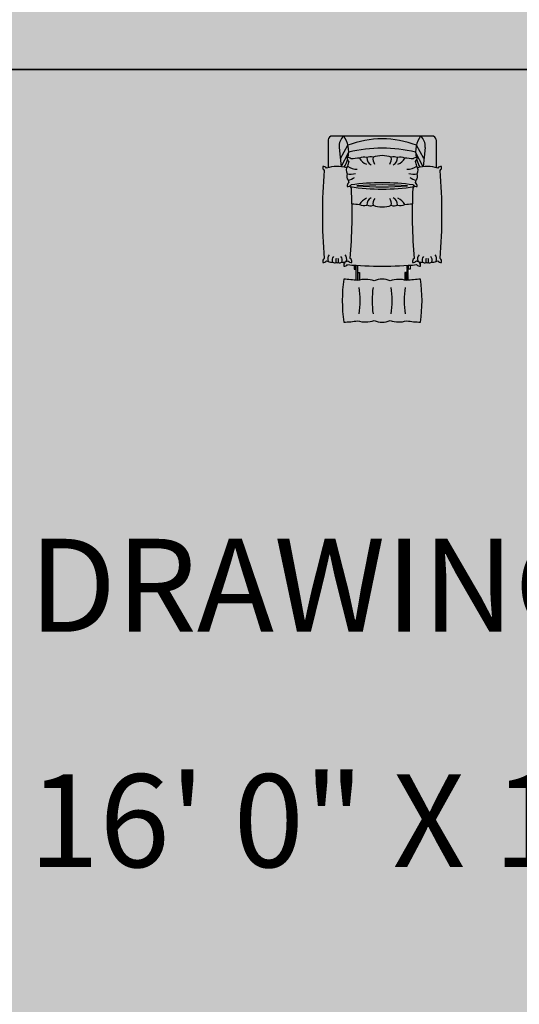
# Model space of a CAD drawing. Units: inches. Extents: x 1704 to 6393, y -157 to 1172.
# Tile 21 of 122: x 2087 to 2161, y 227 to 372. Entities that reach past the tile are written whole.
import ezdxf

# ---------------------------------------------------------------- set-up
doc = ezdxf.new("R2010")
doc.units = ezdxf.units.IN
doc.header["$MEASUREMENT"] = 0
for name, color, linetype, lineweight in [('A-ANNO-DIMS', 7, 'Continuous', 13), ('A-AREA-IDEN', 7, 'Continuous', 18), ('A-FURN', 8, 'Continuous', 18), ('A-WALL-PATT', 7, 'Continuous', 13), ('estofado', 7, 'Continuous', 25), ('WALLS', 7, 'Continuous', 35)]:
    doc.layers.add(name, color=color, linetype=linetype, lineweight=lineweight)
doc.layers.add('A-FLOR-PATT', color=7, linetype='Continuous', lineweight=13, true_color=0xf2f2f2)
doc.styles.get("Standard").update_dxf_attribs({"font": 'arial.ttf'})
doc.dimstyles.get("Standard").update_dxf_attribs({"dimtxt": 6, "dimasz": 2, "dimexe": 0.18, "dimexo": 0.0625, "dimgap": 0.09, "dimtad": 0, "dimtih": 1, "dimtoh": 1, "dimdec": 1, "dimzin": 0, "dimdsep": 46, "dimlunit": 3, "dimtxsty": 'Standard', "dimblk": 'ARCHTICK', "dimcen": 0.09, "dimadec": 0, "dimazin": 0, "dimtfac": 1, "dimtdec": 1, "dimtofl": 0, "dimtmove": 0, "dimatfit": 3, "dimfxl": 1, "dimtolj": 1, "dimtzin": 0, "dimarcsym": 0})

# ---------------------------------------------------------------- blocks, each defined once
blk = doc.blocks.new('Poltrona Del Rey Aliança')
at = {"layer": 'estofado', "ltscale": 0.1}
h = blk.add_hatch(color=256, dxfattribs=at)
h.dxf.hatch_style = 1
h.set_gradient(color1=(204, 209, 209), color2=(140, 151, 151), one_color=1, tint=0.57, name='CYLINDER')
h.paths.add_polyline_path([(-0.3291, -0.0872, -0.258328), (-0.295, 0), (-0.3837, 0, 0.414214), (-0.4137, -0.03), (-0.4137, -0.2425, -0.088666), (-0.3154, -0.2356)])
h.paths.add_polyline_path([(0.4137, -0.03, 0.414214), (0.3837, 0), (0.295, 0, -0.258328), (0.3291, -0.0872), (0.3154, -0.2356, -0.088666), (0.4137, -0.2425)])
h = blk.add_hatch(color=256, dxfattribs=at)
h.dxf.hatch_style = 1
h.set_gradient(color1=(204, 209, 209), color2=(140, 151, 151), one_color=1, tint=0.57, name='INVCYLINDER')
h.paths.add_polyline_path([(0.295, 0), (-0.295, 0, -0.089046), (-0.2635, -0.0705, -0.183028), (0.2635, -0.0705, -0.089046)])
h = blk.add_hatch(color=256, dxfattribs=at)
h.dxf.hatch_style = 1
h.set_gradient(color1=(204, 209, 209), color2=(140, 151, 151), one_color=1, tint=0.57)
h.paths.add_polyline_path([(-0.2635, -0.0705, 0.089046), (-0.295, 0, 0.258328), (-0.3291, -0.0872), (-0.3212, -0.1727)])
h.paths.add_polyline_path([(-0.2571, -0.1231, 0.060804), (-0.2635, -0.0705), (-0.3212, -0.1727), (-0.3154, -0.2356)])
h.paths.add_polyline_path([(-0.2655, -0.1833, -0.142988), (-0.2685, -0.1646, -0.055221), (-0.261, -0.1645, 0.047677), (-0.2571, -0.1231), (-0.3154, -0.2356, -0.022481), (-0.2906, -0.2393, 0.070542)])
h = blk.add_hatch(color=256, dxfattribs=at)
h.dxf.hatch_style = 1
h.set_gradient(color1=(204, 209, 209), color2=(140, 151, 151), one_color=1, tint=0.57, name='INVCYLINDER')
h.paths.add_polyline_path([(-0.2635, -0.0705, -0.060804), (-0.2571, -0.1231, -0.113324), (0.2571, -0.1231, -0.060804), (0.2635, -0.0705, 0.183028)])
h = blk.add_hatch(color=256, dxfattribs=at)
h.dxf.hatch_style = 1
h.set_gradient(color1=(204, 209, 209), color2=(140, 151, 151), one_color=1, tint=0.57)
h.paths.add_polyline_path([(0.295, 0, 0.089046), (0.2635, -0.0705), (0.3211, -0.1738), (0.3291, -0.0872, 0.258328)])
h.paths.add_polyline_path([(0.2635, -0.0705, 0.060804), (0.2571, -0.1231), (0.3154, -0.2356), (0.3211, -0.1738)])
h.paths.add_polyline_path([(0.2571, -0.1231, 0.047677), (0.261, -0.1645, -0.055221), (0.2685, -0.1646, -0.142988), (0.2655, -0.1833, 0.070542), (0.2906, -0.2393, -0.022481), (0.3154, -0.2356)])
h = blk.add_hatch(color=256, dxfattribs=at)
h.dxf.hatch_style = 1
h.set_gradient(color1=(204, 209, 209), color2=(85, 94, 94), one_color=1, tint=0.35, name='CURVED')
h.paths.add_polyline_path([(-0.2568, -0.1947, -0.107782), (-0.2655, -0.1833, -0.070542), (-0.2906, -0.2393, -0.016789), (-0.2722, -0.2436, -0.067663), (-0.2652, -0.2308, -0.033072)])
h.paths.add_polyline_path([(0.2571, -0.1231, 0.113324), (-0.2571, -0.1231, -0.047677), (-0.261, -0.1645, -0.196708), (-0.2383, -0.1763, -0.00792), (-0.1747, -0.1697, -0.182617), (-0.118, -0.1656, -0.204275), (-0.0697, -0.1634, -0.180654), (0.0697, -0.1634, -0.204275), (0.118, -0.1656, -0.182617), (0.1747, -0.1697, -0.00792), (0.2383, -0.1763, -0.196708), (0.261, -0.1645, -0.047677)])
h.paths.add_polyline_path([(0.2655, -0.1833, -0.107782), (0.2568, -0.1947, -0.033072), (0.2652, -0.2308, -0.067663), (0.2722, -0.2436, -0.016789), (0.2906, -0.2393, -0.070542)])
h = blk.add_hatch(color=256, dxfattribs=at)
h.dxf.hatch_style = 1
h.set_gradient(color1=(204, 209, 209), color2=(140, 151, 151), one_color=1, tint=0.57, name='INVCURVED')
h.paths.add_polyline_path([(0.2652, -0.2308, 0.033072), (0.2568, -0.1947, 0.254696), (0.2685, -0.1646, 0.254696), (0.2383, -0.1763, 0.00792), (0.1747, -0.1697, 0.182617), (0.118, -0.1656, 0.187401), (0.0735, -0.1621, 0.016251), (0.0697, -0.1634, 0.180654), (-0.0697, -0.1634, 0.204275), (-0.118, -0.1656, 0.263328), (-0.0893, -0.2185, -0.263328), (-0.118, -0.1656, 0.182617), (-0.1747, -0.1697, 0.00792), (-0.2383, -0.1763, 0.254696), (-0.2685, -0.1646, 0.254696), (-0.2568, -0.1947, 0.033072), (-0.2652, -0.2308, 0.299987), (-0.2685, -0.2905, 0.296972), (-0.2615, -0.3402, 0.016266), (-0.2568, -0.3578, 0.254696), (-0.2685, -0.388, 0.254696), (-0.2383, -0.3763, -0.073513), (0.2383, -0.3763, 0.254696), (0.2685, -0.388, 0.254696), (0.2568, -0.3578, 0.016266), (0.2615, -0.3402, 0.296972), (0.2685, -0.2905, 0.299987)])
h = blk.add_hatch(color=256, dxfattribs=at)
h.dxf.hatch_style = 1
h.set_gradient(color1=(204, 209, 209), one_color=1, tint=1)
h.paths.add_polyline_path([(-0.2358, -0.4039, 0.314303), (-0.2519, -0.386, -0.125347), (-0.2685, -0.388, -0.254696), (-0.2568, -0.3578, -0.016266), (-0.2615, -0.3402, -0.296972), (-0.2685, -0.2905, -0.227702), (-0.2722, -0.2436, 0.140506), (-0.4265, -0.2461, 0.254696), (-0.4567, -0.2344, 0.254696), (-0.445, -0.2646, 0.041763), (-0.445, -0.9409, 0.254696), (-0.4567, -0.971, 0.254696), (-0.4265, -0.9594, 0.011584), (-0.414, -0.9628, 0.212443), (-0.3803, -0.9693, 0.2364), (-0.3527, -0.9714, 0.216836), (-0.3417, -0.9734, 0.091294), (-0.3373, -0.9714, 0.2364), (-0.3097, -0.9693, 0.284493), (-0.3149, -0.9268, -0.284493), (-0.3097, -0.9693, 0.212443), (-0.276, -0.9628, 0.011584), (-0.2635, -0.9594, 0.254696), (-0.2333, -0.971, 0.254696), (-0.245, -0.9409, 0.033141)])
h = blk.add_hatch(color=256, dxfattribs=at)
h.dxf.hatch_style = 1
h.set_gradient(color1=(204, 209, 209), one_color=1, tint=1)
h.paths.add_polyline_path([(0.445, -0.2646, 0.254696), (0.4567, -0.2344, 0.254696), (0.4265, -0.2461, 0.140506), (0.2722, -0.2436, -0.227702), (0.2685, -0.2905, -0.296972), (0.2615, -0.3402, -0.016266), (0.2568, -0.3578, -0.254696), (0.2685, -0.388, -0.125347), (0.2519, -0.386, 0.314303), (0.2358, -0.4039, 0.033141), (0.245, -0.9409, 0.254696), (0.2333, -0.971, 0.254696), (0.2635, -0.9594, 0.011584), (0.276, -0.9628, 0.212443), (0.3097, -0.9693, 0.2364), (0.3373, -0.9714, 0.314353), (0.3527, -0.9714, 0.2364), (0.3803, -0.9693, 0.212443), (0.414, -0.9628, 0.011584), (0.4265, -0.9594, 0.254696), (0.4567, -0.971, 0.254696), (0.445, -0.9409, 0.041763)])
h = blk.add_hatch(color=256, dxfattribs=at)
h.dxf.hatch_style = 1
h.set_gradient(color1=(204, 209, 209), color2=(140, 151, 151), one_color=1, tint=0.57, name='INVCURVED')
h.paths.add_polyline_path([(-0.2383, -0.3763, -0.125347), (-0.2519, -0.386, -0.093275), (-0.2447, -0.3891, 0.075524), (0.2447, -0.3891, -0.093275), (0.2519, -0.386, -0.125347), (0.2383, -0.3763, 0.073513)])
h.paths.add_polyline_path([(0.1958, -0.3832, -0.03688), (-0.1958, -0.3832, -0.03688)], flags=16)
h = blk.add_hatch(color=256, dxfattribs=at)
h.dxf.hatch_style = 1
h.set_gradient(color1=(204, 209, 209), color2=(129, 141, 141), one_color=1, tint=0.53, name='CURVED')
h.paths.add_polyline_path([(0.2356, -0.4071, -0.253895), (0.2447, -0.3891, -0.075524), (-0.2447, -0.3891, -0.253895), (-0.2356, -0.4071, -0.006973), (-0.2317, -0.5201, 0.007144), (-0.1744, -0.5259, -0.00012), (-0.1743, -0.5259, 0.182617), (-0.1176, -0.53, 0.204275), (-0.0693, -0.5322, 0.180654), (0.0701, -0.5322, 0.204275), (0.1184, -0.53, 0.182617), (0.1751, -0.5259, 0.000052), (0.1751, -0.5258, 0.00705), (0.2317, -0.5201, -0.006973)])
h = blk.add_hatch(color=256, dxfattribs=at)
h.dxf.hatch_style = 1
h.set_gradient(color1=(204, 209, 209), one_color=1, tint=1, name='CYLINDER')
h.paths.add_polyline_path([(0.2317, -0.5201, -0.007042), (0.1752, -0.5258, -0.182811), (0.1184, -0.53, -0.204275), (0.0701, -0.5322, -0.180542), (-0.0693, -0.5323, -0.000018), (-0.0694, -0.5323, -0.203561), (-0.1175, -0.53, -0.000024), (-0.1177, -0.53, -0.181815), (-0.1742, -0.5259, -0.007163), (-0.2317, -0.5201, -0.025969), (-0.245, -0.9409, -0.254696), (-0.2333, -0.971, -0.254696), (-0.2635, -0.9594, -0.011584), (-0.276, -0.9628, -0.070407), (-0.2865, -0.9682, 0.130579), (-0.295, -0.9977), (-0.295, -1, 0.254696), (-0.2648, -0.9883, 0.044151), (0.2648, -0.9883, 0.254696), (0.295, -1), (0.295, -0.9977, 0.130579), (0.2865, -0.9682, -0.070407), (0.276, -0.9628, -0.011584), (0.2635, -0.9594, -0.254696), (0.2333, -0.971, -0.254696), (0.245, -0.9409, -0.025969)])
h = blk.add_hatch(color=256, dxfattribs=at)
h.dxf.hatch_style = 1
h.set_gradient(color1=(204, 209, 209), one_color=1, tint=1, name='CYLINDER')
h.paths.add_polyline_path([(0.295, -1.0999, 0.031185), (0.1884, -1.1106, 0.17196), (0.0623, -1.1138, 0.223433), (-0.0623, -1.1138, 0.17196), (-0.1884, -1.1106, 0.031185), (-0.295, -1.0999, 0.066975), (-0.295, -1.43, 0.031185), (-0.1884, -1.4193, 0.17196), (-0.0623, -1.4161, 0.223433), (0.0623, -1.4161, 0.17196), (0.1884, -1.4193, 0.031185), (0.295, -1.43, 0.066975)])
at = {"layer": 'estofado'}
for p, q in [((0.3837, 0), (-0.3837, 0)), ((-0.4137, -0.03), (-0.4137, -0.2425)), ((0.4137, -0.03), (0.4137, -0.2425)), ((-0.3291, -0.0872), (-0.3154, -0.2356)), ((0.3291, -0.0872), (0.3154, -0.2356)), ((-0.295, -0.9701), (-0.295, -1)), ((0.295, -1), (0.295, -0.9701))]:
    blk.add_line(p, q, dxfattribs=at)
at = {"layer": 'estofado', "ltscale": 0.1}
for p, q in [((-0.3212, -0.1727), (-0.2635, -0.0705)), ((0.3211, -0.1738), (0.2635, -0.0705)), ((-0.3154, -0.2356), (-0.2571, -0.1231)), ((0.3154, -0.2356), (0.2571, -0.1231))]:
    blk.add_line(p, q, dxfattribs=at)
for points in [[(-0.2141, -0.9924), (-0.2141, -1.0234), (-0.2033, -1.0234), (-0.2033, -0.9931)], [(-0.2003, -1.1087), (-0.2003, -0.9933)], [(-0.1897, -0.994), (-0.1897, -1.1104)], [(-0.1852, -1.1096), (-0.1852, -1.0474), (-0.1745, -1.0474), (-0.1745, -1.1066)], [(0.1852, -1.1096), (0.1852, -1.0474), (0.1745, -1.0474), (0.1745, -1.1066)], [(0.1897, -0.994), (0.1897, -1.1104)], [(0.2003, -1.1087), (0.2003, -0.9933)], [(0.2141, -0.9924), (0.2141, -1.0234), (0.2033, -1.0234), (0.2033, -0.9931)]]:
    blk.add_lwpolyline(points, dxfattribs=at)
at = {"layer": 'estofado'}
for centre, radius, start, end in [((-0.3837, -0.03), 0.03, 90, 180), ((-0.2333, -0.0744), 0.0967, 129.65366, 187.59148), ((-0.4756, -0.1231), 0.2185, 349.08151, 34.27248), ((0.4756, -0.1231), 0.2185, 145.72752, 190.91849), ((0.2333, -0.0744), 0.0967, 352.40852, 50.34634), ((0.3837, -0.03), 0.03, 360, 90), ((-0.4756, -0.1231), 0.2185, 327.85602, 343.99631), ((-0.2349, -0.1689), 0.0338, 172.61866, 229.77535), ((-0.2641, -0.1981), 0.0338, 40.22465, 97.38134), ((0.0111, -0.2763), 0.28, 163.06826, 170.64501), ((0, -2.1798), 2.0176, 94.96806, 96.78307), ((0, -2.1798), 2.0176, 83.21693, 85.03194), ((0.2641, -0.1981), 0.0338, 82.61866, 139.77535), ((0.2349, -0.1689), 0.0338, 310.22465, 7.38134), ((-0.0111, -0.2763), 0.28, 9.35499, 16.93174), ((0.4756, -0.1231), 0.2185, 196.00369, 212.14398), ((3.5965, -0.6027), 4.0556, 175.21711, 184.78289), ((-0.4232, -0.2388), 0.0338, 172.61866, 229.77535), ((-0.4524, -0.268), 0.0338, 40.22465, 97.38134), ((-0.345, -0.514), 0.28, 74.93962, 106.93174), ((-0.2215, -0.2632), 0.0544, 143.38498, 210.17914), ((-0.2269, -0.31), 0.046, 154.98172, 221.1415), ((0.2269, -0.31), 0.046, 318.8585, 25.01828), ((0.2215, -0.2632), 0.0544, 329.82086, 36.61502), ((0.345, -0.514), 0.28, 73.06826, 105.06038), ((0.4524, -0.268), 0.0338, 82.61866, 139.77535), ((0.4232, -0.2388), 0.0338, 310.22465, 7.38134), ((-3.5965, -0.6027), 4.0556, 355.21711, 4.78289), ((-0.2349, -0.3836), 0.0338, 130.22465, 187.38134), ((-0.2641, -0.3545), 0.0338, 262.61866, 319.77535), ((0.0111, -0.2763), 0.28, 193.20412, 196.93174), ((0, -3.0337), 2.6577, 85.77582, 94.22418), ((0.2641, -0.3545), 0.0338, 220.22465, 277.38134), ((-0.0111, -0.2763), 0.28, 343.06826, 346.79588), ((0.2349, -0.3836), 0.0338, 352.61866, 49.77535), ((-0.2567, -0.4065), 0.0211, 358.53397, 76.83372), ((-4.2865, -0.6027), 4.0556, 355.21711, 2.80978), ((0, 2.2673), 2.6577, 265.77582, 274.22418), ((4.2865, -0.6027), 4.0556, 177.19022, 184.78289), ((0.2567, -0.4065), 0.0211, 103.16628, 181.46603), ((0, 1.4842), 2.0176, 263.40516, 265.04688), ((0, 1.4842), 2.0176, 274.97902, 276.59484), ((0, 1.4842), 2.0176, 266.65527, 266.66071), ((0, 1.4842), 2.0176, 268.02834, 268.03255), ((-0.4232, -0.9667), 0.0338, 130.22465, 187.38134), ((-0.4524, -0.9375), 0.0338, 262.61866, 319.77535), ((-0.345, -0.6915), 0.28, 253.06826, 255.723), ((-0.2353, -0.9988), 0.0598, 149.12344, 181.11851), ((-0.345, -0.6915), 0.28, 284.277, 286.93174), ((-0.2376, -0.9375), 0.0338, 220.22465, 277.38134), ((-0.2668, -0.9667), 0.0338, 352.61866, 49.77535), ((0.2668, -0.9667), 0.0338, 130.22465, 187.38134), ((0.2376, -0.9375), 0.0338, 262.61866, 319.77535), ((0.345, -0.6915), 0.28, 253.06826, 255.723), ((0.2353, -0.9988), 0.0598, 358.88149, 30.87656), ((0.345, -0.6915), 0.28, 284.277, 286.93174), ((0.4524, -0.9375), 0.0338, 220.22465, 277.38134), ((0.4232, -0.9667), 0.0338, 352.61866, 49.77535), ((-0.2907, -0.9665), 0.0338, 262.61866, 319.77535), ((0, 2.0052), 3.0052, 264.94391, 275.05609), ((0.2907, -0.9665), 0.0338, 220.22465, 277.38134)]:
    blk.add_arc(centre, radius, start, end, dxfattribs=at)
at = {"layer": 'estofado', "ltscale": 0.1}
for centre, radius, start, end in [((0, -0.7661), 0.7439, 69.25617, 110.74383), ((0, -1.2427), 1.1487, 77.06919, 102.93081), ((0, -0.3501), 0.1993, 69.51952, 110.48048), ((-0.1409, -0.2427), 0.0805, 73.46231, 114.85878), ((-0.0792, -0.1148), 0.1102, 209.89617, 247.80825), ((-0.0912, -0.2211), 0.0616, 69.57655, 115.75748), ((-0.057, -0.1667), 0.061, 178.98456, 242.48365), ((-0.0035, -0.1761), 0.0675, 169.12551, 216.59576), ((0.0035, -0.1761), 0.0675, 323.40424, 10.87449), ((0.0912, -0.2211), 0.0616, 64.24252, 110.42345), ((0.057, -0.1667), 0.061, 297.51635, 1.01544), ((0.1409, -0.2427), 0.0805, 65.14122, 106.53769), ((0.0792, -0.1148), 0.1102, 292.19175, 330.10383), ((-0.2431, -0.1831), 0.1104, 256.68043, 289.83371), ((-0.2036, -0.1635), 0.0913, 227.53176, 278.05529), ((0.2036, -0.1635), 0.0913, 261.94471, 312.46824), ((0.2431, -0.1831), 0.1104, 250.16629, 283.31957), ((-0.3064, -0.1722), 0.1739, 284.94614, 302.97426), ((0, -1.9883), 1.6296, 81.59117, 98.40883), ((0.3064, -0.1722), 0.1739, 237.02574, 255.05386), ((0, 1.222), 1.6296, 261.36198, 278.63802), ((-0.0788, -0.5808), 0.1102, 112.19175, 150.10383), ((-0.1405, -0.4529), 0.0805, 245.14122, 286.53769), ((-0.0566, -0.5289), 0.061, 117.51635, 181.01544), ((-0.0031, -0.5195), 0.0675, 143.40424, 190.87449), ((0.0039, -0.5195), 0.0675, 349.12551, 36.59576), ((0.0574, -0.5289), 0.061, 358.98456, 62.48365), ((0.1413, -0.4529), 0.0805, 253.46231, 294.85878), ((0.0796, -0.5808), 0.1102, 29.89617, 67.80825), ((-0.0908, -0.4745), 0.0616, 244.24252, 290.42345), ((0.0004, -0.3455), 0.1993, 249.51952, 290.48048), ((0.0916, -0.4745), 0.0616, 249.57655, 295.75748), ((-0.369, -0.9438), 0.0489, 140.1555, 202.877), ((-0.3899, -0.9281), 0.0423, 235.25652, 283.23173), ((-0.3434, -0.9522), 0.0406, 137.80589, 204.86284), ((-0.3644, -0.9429), 0.0308, 238.98878, 292.19094), ((-0.3124, -0.9555), 0.0434, 159.33684, 201.47674), ((-0.345, -0.9603), 0.0135, 235.09864, 304.90136), ((-0.3776, -0.9555), 0.0434, 338.52326, 20.66316), ((-0.3256, -0.9429), 0.0308, 247.80906, 301.01122), ((-0.3466, -0.9522), 0.0406, 335.13716, 42.19411), ((-0.3001, -0.9281), 0.0423, 256.76827, 304.74348), ((-0.321, -0.9438), 0.0489, 337.123, 39.8445), ((0.321, -0.9438), 0.0489, 140.1555, 202.877), ((0.3001, -0.9281), 0.0423, 235.25652, 283.23173), ((0.3466, -0.9522), 0.0406, 137.80589, 204.86284), ((0.3256, -0.9429), 0.0308, 238.98878, 292.19094), ((0.3776, -0.9555), 0.0434, 159.33684, 201.47674), ((0.345, -0.9603), 0.0135, 235.09864, 304.90136), ((0.3124, -0.9555), 0.0434, 338.52326, 20.66316), ((0.3644, -0.9429), 0.0308, 247.80906, 301.01122), ((0.3434, -0.9522), 0.0406, 335.13716, 42.19411), ((0.3899, -0.9281), 0.0423, 256.76827, 304.74348), ((0.369, -0.9438), 0.0489, 337.123, 39.8445), ((0.9317, -1.2649), 1.2378, 172.33668, 187.66332), ((-0.3276, -1.9587), 0.8594, 80.68246, 87.82718), ((-0.1299, -1.2902), 0.1889, 69.03471, 108.06338), ((0, -1.2462), 0.1463, 64.81025, 115.18975), ((0.1299, -1.2902), 0.1889, 71.93662, 110.96529), ((0.3276, -1.9587), 0.8594, 92.17282, 99.31754), ((-0.9317, -1.2649), 1.2378, 352.33668, 7.66332), ((-0.8046, -1.2649), 0.6352, 350.72425, 9.27575), ((0.7218, -1.2649), 0.7985, 172.63295, 187.36705), ((-0.7218, -1.2649), 0.7985, 352.63295, 7.36705), ((0.8046, -1.2649), 0.6352, 170.72425, 189.27575), ((-0.3276, -0.5712), 0.8594, 272.17282, 279.31754), ((-0.1299, -1.2397), 0.1889, 251.93662, 290.96529), ((0, -1.2837), 0.1463, 244.81025, 295.18975), ((0.1299, -1.2397), 0.1889, 249.03471, 288.06338), ((0.3276, -0.5712), 0.8594, 260.68246, 267.82718)]:
    blk.add_arc(centre, radius, start, end, dxfattribs=at)
blk = doc.blocks.new('_ArchTick')
at = {"color": 0, "linetype": 'ByBlock', "const_width": 0.15}
blk.add_lwpolyline([(-0.5, -0.5), (0.5, 0.5)], dxfattribs=at)
blk = doc.blocks.new('*D93')
at = {"layer": 'A-ANNO-DIMS', "color": 0, "lineweight": -2, "transparency": 16777216}
for p, q in [((2605.29, 895.21), (1829.7, 895.21)), ((1829.88, 895.21), (1829.88, 495.87)), ((1829.88, 90.21), (1829.88, 489.56)), ((2605.29, 90.21), (1829.7, 90.21))]:
    blk.add_line(p, q, dxfattribs=at)
at = {"layer": 'Defpoints', "color": 0, "lineweight": -3, "transparency": 16777216}
for p in [(2605.35, 895.21), (1829.88, 90.21), (2605.35, 90.21)]:
    blk.add_point(p, dxfattribs=at)
at = {"layer": 'A-ANNO-DIMS', "color": 0, "lineweight": -2, "transparency": 16777216, "xscale": 2, "yscale": 2, "zscale": 2}
for p, rotation in [((1829.88, 895.21), 90), ((1829.88, 90.21), 270)]:
    blk.add_blockref('_ArchTick', p, dxfattribs=dict(at, rotation=rotation))
at = {"layer": 'A-ANNO-DIMS', "color": 0, "transparency": 16777216, "insert": (1829.88, 492.71), "char_height": 6, "attachment_point": 5}
blk.add_mtext('\\A1;805', dxfattribs=at)

msp = doc.modelspace()

# ---------------------------------------------------------------- hatches: boundary and pattern name
at = {"layer": 'A-FLOR-PATT', "transparency": 33554528}
h = msp.add_hatch(color=256, dxfattribs=at)
h.dxf.hatch_style = 1
h.paths.add_polyline_path([(2273.349, 538.213), (2081.349, 538.213), (2081.349, 372.213), (2273.349, 372.213)])
h.paths.add_polyline_path([(2189.542, 505.951), (2184.316, 505.951), (2184.316, 505.591), (2169.442, 505.591), (2169.442, 505.951), (2164.216, 505.951, -0.4142136), (2163.814, 506.353), (2163.814, 526.093, -0.4142136), (2164.216, 526.495), (2189.542, 526.495, -0.4142136), (2189.944, 526.093), (2189.944, 506.353, -0.4142136)], flags=16)
h.paths.add_polyline_path([(2200.535, 511.491), (2200.535, 526.191), (2217.621, 526.191), (2217.621, 511.491), (2214.605, 511.491, -0.3946213), (2214.203, 511.116), (2203.952, 511.116, -0.3946213), (2203.551, 511.491)], flags=16)
h.paths.add_polyline_path([(2200.736, 511.692), (2200.736, 525.99), (2203.55, 525.99), (2203.55, 523.838, 0.1045605), (2214.605, 523.838), (2214.605, 525.99), (2217.42, 525.99), (2217.42, 511.692), (2214.605, 511.692), (2214.605, 523.838, -0.1045605), (2203.55, 523.838), (2203.55, 511.692)], flags=0)
h.paths.add_polyline_path([(2203.952, 511.317, -0.4142136), (2203.751, 511.518), (2203.751, 523.591, 0.099912), (2214.404, 523.591), (2214.404, 511.518, -0.4142136), (2214.203, 511.317)], flags=0)
h.paths.add_polyline_path([(2184.084, 516.015, -0.0686795), (2169.674, 516.015), (2169.674, 522.073), (2184.084, 522.073)], flags=0)
h.paths.add_polyline_path([(2183.325, 518.606, -0.0772766), (2170.433, 518.606), (2170.433, 521.123, -0.0235462), (2183.325, 521.123)], flags=0)
h.paths.add_polyline_path([(2135.029, 507.225, -0.1405189), (2135.191, 507.834, -0.0513838), (2135.029, 507.797)], flags=16)
h.paths.add_polyline_path([(2146.318, 498.997, -0.0311848), (2144.279, 499.202, -0.1719602), (2141.865, 499.263, -0.2234326), (2139.482, 499.263, -0.1719602), (2137.068, 499.202, -0.0311848), (2135.029, 498.997, -0.066975), (2135.029, 505.313, -0.0276914), (2136.841, 505.144), (2136.841, 506.777), (2136.576, 506.777), (2136.576, 507.371, 0.039911), (2145.741, 507.448, 0.2546956), (2146.318, 507.225), (2146.318, 507.269, 0.1305786), (2146.156, 507.834, -0.0704067), (2145.953, 507.935, -0.011584), (2145.714, 508.002, -0.2546956), (2145.137, 507.779, -0.2546956), (2145.361, 508.355, -0.0259693), (2145.107, 516.407, -0.0070422), (2144.025, 516.297, -0.1828112), (2142.939, 516.218, -0.2042746), (2142.015, 516.175, -0.1805419), (2139.348, 516.174, -0.0000184), (2139.345, 516.174, -0.2035615), (2138.425, 516.217, -0.0000237), (2138.421, 516.217, -0.1818152), (2137.34, 516.296, -0.0071635), (2136.24, 516.407, 0.007166), (2136.162, 518.63, 0.314303), (2135.854, 518.974, -0.1253469), (2135.537, 518.935, -0.2546956), (2135.76, 519.512, -0.0162662), (2135.67, 519.849, -0.296972), (2135.535, 520.8, -0.227702), (2135.464, 521.698, 0.1283977), (2132.757, 521.718), (2132.757, 525.785, -0.4142136), (2133.331, 526.359), (2148.015, 526.359, -0.4142136), (2148.589, 525.785), (2148.589, 521.718, -0.0118936), (2148.835, 521.65, -0.2546956), (2149.412, 521.873, -0.2546956), (2149.188, 521.296, -0.0417628), (2149.188, 508.355, -0.2546956), (2149.412, 507.779, -0.2546956), (2148.835, 508.002, -0.011584), (2148.596, 507.935, -0.2124435), (2147.949, 507.813, -0.2363999), (2147.423, 507.772, -0.3143526), (2147.126, 507.772, -0.2363999), (2146.6, 507.813, -0.0879275), (2146.318, 507.797), (2146.318, 507.225, -0.2546956), (2145.741, 507.448, -0.0042329), (2144.771, 507.371), (2144.771, 506.777), (2144.506, 506.777), (2144.506, 505.144, -0.0276914), (2146.318, 505.313, -0.066975)], flags=16)
h.paths.add_polyline_path([(2141.865, 505.047, 0.2234326), (2139.482, 505.047, 0.1738145), (2137.043, 505.1), (2137.043, 506.317), (2137.335, 506.317), (2137.335, 505.184, -0.1522072), (2139.482, 505.047, -0.2234326), (2141.865, 505.047, -0.1522072), (2144.011, 505.184), (2144.011, 506.317), (2144.304, 506.317), (2144.304, 505.1, 0.1738145)], flags=0)
h.paths.add_polyline_path([(2145.233, 522.986, 0.0079197), (2144.017, 523.111, 0.1826165), (2142.931, 523.19, 0.2042746), (2142.008, 523.233, 0.1806536), (2139.339, 523.233, 0.2042746), (2138.415, 523.19, 0.1826165), (2137.33, 523.111, 0.0079197), (2136.114, 522.986, 0.1967082), (2135.679, 523.212, 0.047677), (2135.755, 524.004), (2134.638, 521.852), (2134.376, 524.691, -0.2583282), (2135.029, 526.359, -0.0890464), (2135.632, 525.01, -0.1830277), (2145.715, 525.01, -0.0890464), (2146.318, 526.359, -0.2583282), (2146.971, 524.691), (2146.709, 521.852), (2145.592, 524.004, 0.047677), (2145.668, 523.212, 0.1967082)], flags=0)
h.paths.add_polyline_path([(2144.419, 519.027, -0.0368796), (2136.927, 519.027, -0.0368796)], flags=0)
h.paths.add_polyline_path([(2273.349, 629.213), (2213.349, 629.213), (2213.349, 573.213), (2213.349, 545.213), (2273.349, 545.213)])
h.paths.add_polyline_path([(2273.349, 711.213), (2207.349, 711.213), (2207.349, 709.213), (2231.349, 709.213), (2231.349, 707.213), (2207.349, 707.213), (2207.349, 631.213), (2273.349, 631.213)])
h.paths.add_polyline_path([(2273.349, 364.213), (2081.349, 364.213), (2081.349, 202.213), (2225.349, 202.213), (2229.181, 202.213), (2230.482, 202.213), (2268.215, 202.213), (2269.516, 202.213), (2273.349, 202.213)])
h.paths.add_polyline_path([(2203.551, 339.558, 0.3946213), (2203.952, 339.183), (2214.203, 339.183), (2214.203, 339.384), (2203.751, 339.384), (2203.751, 339.558)], flags=16)
h.paths.add_polyline_path([(2203.55, 351.7), (2203.55, 339.759), (2200.535, 339.759), (2200.535, 354.258), (2217.621, 354.258), (2217.621, 339.558), (2214.404, 339.558), (2214.404, 351.659, -0.101837)], flags=16)
h.paths.add_polyline_path([(2214.404, 354.057), (2214.605, 354.057), (2214.605, 354.258), (2214.404, 354.258)], flags=16)
h.paths.add_polyline_path([(2189.542, 334.018), (2184.316, 334.018), (2184.316, 333.658), (2169.442, 333.658), (2169.442, 334.018), (2164.216, 334.018, -0.4142136), (2163.814, 334.42), (2163.814, 354.161, -0.4142136), (2164.216, 354.563), (2189.542, 354.563, -0.4142136), (2189.944, 354.161), (2189.944, 334.42, -0.4142136)], flags=16)
h.paths.add_polyline_path([(2184.084, 344.083, -0.0686795), (2169.674, 344.083), (2169.674, 349.85), (2165.7, 350.14), (2188.058, 350.14), (2184.084, 349.85)], flags=0)
h.paths.add_polyline_path([(2183.325, 346.673, -0.0772766), (2170.433, 346.673), (2170.433, 349.19, -0.0235462), (2183.325, 349.19)], flags=0)
h.paths.add_polyline_path([(2134.638, 349.919), (2134.376, 352.758, -0.2583282), (2135.029, 354.426), (2133.331, 354.426, 0.4142136), (2132.757, 353.852), (2132.757, 349.785, -0.0886664)], flags=16)
h.paths.add_polyline_path([(2136.114, 351.053, -0.0079197), (2137.33, 351.178, -0.1826165), (2138.415, 351.257, -0.2042746), (2139.339, 351.3, -0.1806536), (2142.008, 351.3, -0.2042746), (2142.931, 351.257, -0.1826165), (2144.017, 351.178, -0.0079197), (2145.233, 351.053, -0.1967082), (2145.668, 351.279, -0.047677), (2145.592, 352.071, 0.1133241), (2135.755, 352.071, -0.047677), (2135.679, 351.279, -0.1967082)], flags=16)
h.paths.add_polyline_path([(2145.184, 346.697, 0.0331414), (2145.361, 336.423, 0.2546956), (2145.137, 335.846, 0.3030408), (2145.781, 336.164, 0.2903634), (2146.6, 335.88, 0.2363999), (2147.126, 335.839, -0.280712), (2147.275, 336.69, -0.280712), (2147.423, 335.839, 0.2363999), (2147.949, 335.88, 0.2903634), (2148.768, 336.164, 0.3030408), (2149.412, 335.846, 0.2546956), (2149.188, 336.423, 0.0417628), (2149.188, 349.363, 0.2546956), (2149.412, 349.94, 0.2546956), (2148.835, 349.717, 0.1405058), (2145.883, 349.765, -0.227702), (2145.812, 348.867, -0.296972), (2145.677, 347.916, -0.0162662), (2145.586, 347.579, -0.2546956), (2145.81, 347.002, -0.1253469), (2145.493, 347.041, 0.314303)], flags=16)
h.paths.add_polyline_path([(2135.029, 335.292, -0.1405189), (2135.191, 335.901, -0.1399435), (2134.747, 335.88, -0.2363999), (2134.22, 335.839, -0.3143526), (2133.924, 335.839, -0.280712), (2134.072, 336.69, -0.280712), (2134.22, 335.839, 0.2363999), (2134.747, 335.88, 0.2903634), (2135.566, 336.164, 0.3030408), (2136.209, 335.846, 0.2546956), (2135.985, 336.423, 0.0331414), (2136.162, 346.697, 0.314303), (2135.854, 347.041, -0.1253469), (2135.537, 347.002, -0.2546956), (2135.76, 347.579, -0.0162662), (2135.67, 347.916, -0.296972), (2135.535, 348.867, -0.2999866), (2135.599, 350.01, -0.0330719), (2135.76, 350.7, -0.3502076), (2135.604, 351.492), (2134.638, 349.919), (2135.604, 351.492, 0.3502076), (2135.76, 350.7, 0.0330719), (2135.599, 350.01, 0.2999866), (2135.535, 348.867, 0.296972), (2135.67, 347.916, 0.0279375), (2135.971, 347.698, 0.3576436), (2135.537, 347.002, 0.1253469), (2135.854, 347.041, -0.3555912), (2136.165, 346.637, -0.0329482), (2135.985, 336.423, -0.2546956), (2136.209, 335.846, -0.2546956), (2135.632, 336.069, -0.011584), (2135.393, 336.003, -0.1222327), (2135.029, 335.864)], flags=16)
h.paths.add_polyline_path([(2136.841, 335.42), (2136.783, 335.423), (2136.783, 334.844), (2136.841, 334.471)], flags=16)
h.paths.add_polyline_path([(2146.318, 327.064, -0.0311848), (2144.279, 327.269, -0.1719602), (2141.865, 327.33, -0.2234326), (2139.482, 327.33, -0.1719602), (2137.068, 327.269, -0.0311848), (2135.029, 327.064, -0.066975), (2135.029, 333.38, -0.0311848), (2137.068, 333.175, -0.1719602), (2139.482, 333.114, -0.2234326), (2141.865, 333.114, -0.1522072), (2144.011, 333.251), (2144.011, 334.384), (2144.304, 335.406, 0.0020345), (2144.771, 335.438), (2144.771, 334.844), (2144.506, 333.211, -0.0276914), (2146.318, 333.38, -0.066975)], flags=16)
h.paths.add_polyline_path([(2137.129, 334.384), (2137.335, 334.384), (2137.335, 333.251), (2137.129, 333.195)], flags=16)
h.paths.add_polyline_path([(2144.419, 347.094, -0.0368796), (2136.927, 347.094, -0.0368796)], flags=16)
at = {"layer": 'A-WALL-PATT', "transparency": 33554643}
h = msp.add_hatch(color=256, dxfattribs=at)
h.dxf.hatch_style = 1
h.paths.add_polyline_path([(2167.349, 895.213), (2073.349, 895.213), (2073.349, 887.213), (2081.349, 887.213), (2167.349, 887.213)])
h.paths.add_polyline_path([(2465.349, 895.213), (2273.349, 895.213), (2273.349, 903.213), (2263.349, 903.213), (2263.349, 895.213), (2263.349, 887.213), (2325.349, 887.213), (2325.349, 863.213), (2333.349, 863.213), (2333.349, 887.213), (2465.349, 887.213)])
h.paths.add_polyline_path([(2533.349, 895.213), (2513.349, 895.213), (2513.349, 887.213), (2513.349, 861.213), (2517.349, 861.213), (2517.349, 887.213), (2533.349, 887.213)])
h.paths.add_polyline_path([(2605.349, 895.213), (2581.349, 895.213), (2581.349, 887.213), (2597.349, 887.213), (2597.349, 854.213), (2605.349, 854.213)])
h.paths.add_polyline_path([(2605.349, 752.213), (2629.349, 752.213), (2629.349, 716.213), (2605.349, 716.213), (2605.349, 712.213), (2719.349, 712.213), (2719.349, 716.213), (2631.349, 716.213), (2631.349, 754.213), (2605.349, 754.213), (2605.349, 794.213), (2597.349, 794.213), (2597.349, 787.213), (2517.349, 787.213), (2517.349, 813.213), (2513.349, 813.213), (2513.349, 783.213), (2517.349, 783.213), (2597.349, 783.213), (2597.349, 719.213), (2517.349, 719.213), (2517.349, 753.213), (2513.349, 753.213), (2513.349, 719.213), (2365.349, 719.213), (2365.349, 763.213), (2325.349, 763.213), (2325.349, 755.213), (2357.349, 755.213), (2357.349, 719.213), (2325.349, 719.213), (2325.349, 711.213), (2547.349, 711.213), (2547.349, 615.213), (2449.349, 615.213), (2449.349, 607.213), (2514.349, 607.213), (2514.349, 546.213), (2439.349, 546.213), (2425.349, 546.213), (2425.349, 607.213), (2425.349, 615.213), (2350.349, 615.213), (2350.349, 589.713), (2358.349, 589.713), (2358.349, 610.213), (2420.349, 610.213), (2420.349, 545.213), (2358.349, 545.213), (2358.349, 565.713), (2350.349, 565.713), (2350.349, 538.213), (2469.349, 538.213), (2469.349, 459.213), (2469.349, 372.213), (2423.349, 372.213), (2423.349, 364.213), (2473.349, 364.213), (2473.349, 318.213), (2477.349, 318.213), (2477.349, 364.213), (2547.349, 364.213), (2547.349, 352.213), (2549.349, 352.213), (2549.349, 364.213), (2597.349, 364.213), (2597.349, 328.213), (2549.349, 328.213), (2547.349, 328.213), (2547.349, 326.213), (2549.349, 326.213), (2597.349, 326.213), (2605.349, 326.213), (2605.349, 377.057), (2597.349, 377.057), (2597.349, 372.213), (2477.349, 372.213), (2477.349, 451.213), (2597.349, 451.213), (2605.349, 451.213), (2605.349, 459.213), (2597.349, 459.213), (2477.349, 459.213), (2477.349, 538.213), (2597.349, 538.213), (2597.349, 495.213), (2605.349, 495.213), (2605.349, 512.213), (2631.349, 512.213), (2631.349, 568.213), (2605.349, 568.213), (2605.349, 577.213), (2597.349, 577.213), (2597.349, 542.213), (2518.349, 542.213), (2518.349, 607.213), (2532.349, 607.213), (2605.349, 607.213), (2605.349, 615.213), (2597.349, 615.213), (2551.349, 615.213), (2551.349, 711.213), (2597.349, 711.213), (2597.349, 645.213), (2605.349, 645.213), (2605.349, 712.213), (2605.349, 716.213)])
h.paths.add_polyline_path([(2605.349, 566.213), (2629.349, 566.213), (2629.349, 514.213), (2605.349, 514.213)], flags=16)
h.paths.add_polyline_path([(2381.349, 372.213), (2349.349, 372.213), (2349.349, 202.213), (2337.349, 202.213), (2337.349, 194.213), (2349.349, 194.213), (2349.349, 90.213), (2349.349, 72.213), (2357.349, 72.213), (2357.349, 90.213), (2381.349, 90.213), (2381.349, 98.213), (2357.349, 98.213), (2357.349, 266.213), (2381.349, 266.213), (2381.349, 270.213), (2353.349, 270.213), (2353.349, 364.213), (2381.349, 364.213)])
h.paths.add_polyline_path([(2605.349, 302.213), (2597.349, 302.213), (2597.349, 270.213), (2477.349, 270.213), (2477.349, 294.213), (2473.349, 294.213), (2473.349, 270.213), (2423.349, 270.213), (2423.349, 266.213), (2597.349, 266.213), (2597.349, 218.213), (2605.349, 218.213)])
h.paths.add_polyline_path([(2605.349, 146.213), (2597.349, 146.213), (2597.349, 98.213), (2429.349, 98.213), (2429.349, 90.213), (2597.349, 90.213), (2597.349, 72.213), (2605.349, 72.213), (2605.349, 90.213)])
h.paths.add_polyline_path([(2225.349, 202.213), (2049.349, 202.213), (2049.349, 194.213), (2225.349, 194.213)])
h.paths.add_polyline_path([(2289.349, 202.213), (2277.349, 202.213), (2273.349, 202.213), (2269.516, 202.213), (2269.516, 194.213), (2273.349, 194.213), (2277.349, 194.213), (2289.349, 194.213)])
h.paths.add_polyline_path([(2273.349, 372.213), (2029.19, 372.213), (2029.19, 364.213), (2273.349, 364.213)])
h.paths.add_polyline_path([(2277.349, 545.213), (2213.349, 545.213), (2213.349, 573.213), (2205.349, 573.213), (2177.349, 573.213), (2177.349, 545.213), (2073.349, 545.213), (2073.349, 538.213), (2081.349, 538.213), (2277.349, 538.213)])
h.paths.add_polyline_path([(2181.349, 545.213), (2181.349, 569.213), (2205.349, 569.213), (2205.349, 545.213)], flags=16)
h.paths.add_polyline_path([(2277.349, 719.213), (2081.349, 719.213), (2073.349, 719.213), (2073.349, 711.213), (2154.575, 711.213), (2205.349, 711.213), (2205.349, 687.213), (2205.349, 629.213), (2213.349, 629.213), (2273.349, 629.213), (2273.349, 631.213), (2207.349, 631.213), (2207.349, 707.213), (2231.349, 707.213), (2231.349, 709.213), (2207.349, 709.213), (2207.349, 711.213), (2277.349, 711.213)])

# ---------------------------------------------------------------- linework, layer by layer
at = {"layer": 'WALLS'}
msp.add_line((2277.349, 364.213), (2029.19, 364.213), dxfattribs=at)

# ---------------------------------------------------------------- block references
at = {"layer": 'A-FURN', "xscale": 19.13431682689143, "yscale": 19.13431682689143, "zscale": 19.13431682689143}
msp.add_blockref('Poltrona Del Rey Aliança', (2140.673, 354.426), dxfattribs=at)

# ---------------------------------------------------------------- texts
at = {"layer": 'A-ANNO-DIMS'}
msp.add_text('16\' 0" X 13\' 6"', height=13.6672, dxfattribs=at).set_placement((2088.773, 246.952))
at = {"layer": 'A-AREA-IDEN'}
msp.add_text('DRAWING ROOM', height=13.6672, dxfattribs=at).set_placement((2088.773, 281.553))

# ---------------------------------------------------------------- dimensions: what is measured, and where the dimension line sits
at = {"layer": 'A-ANNO-DIMS'}
dim = msp.add_linear_dim(base=(1829.878, 90.213), p1=(2605.349, 895.213), p2=(2605.349, 90.213), angle=90, dimstyle='Standard', override={"dimdec": 0, "dimlfac": 1, "dimrnd": 0, "dimzin": 0, "dimdsep": 46, "dimlunit": 2}, dxfattribs=at)
dim.commit()
dim.dimension.update_dxf_attribs({"geometry": '*D93', "text_midpoint": (1829.878, 492.713)})

doc.saveas('drawing.dxf')
